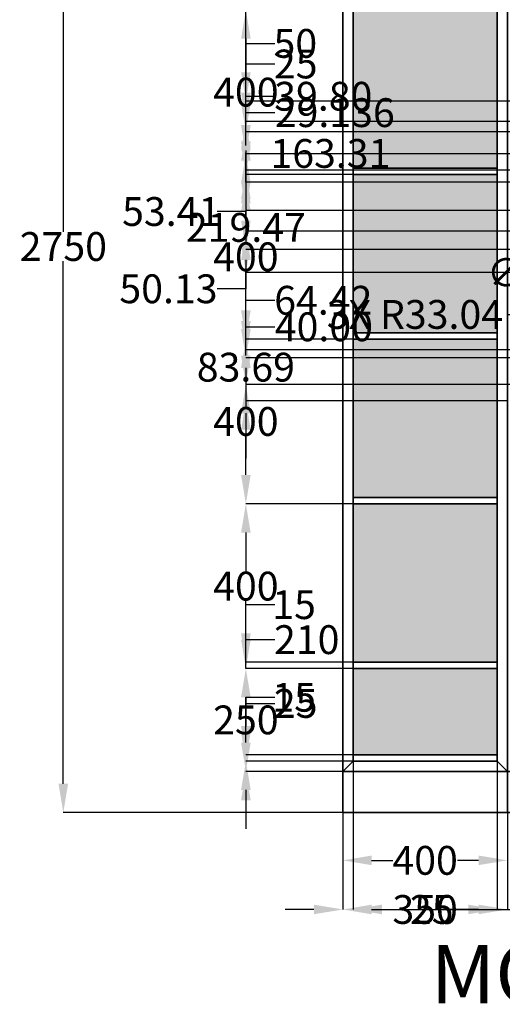
# Model space of a CAD drawing. Units: inches. Extents: x 600 to 5582, y -464 to 3142.
# Tile 1 of 9: x 600 to 1772, y -464 to 1928. Entities that reach past the tile are written whole.
import ezdxf

# ---------------------------------------------------------------- set-up
doc = ezdxf.new("R2010")
doc.units = ezdxf.units.IN
doc.header["$MEASUREMENT"] = 0
for name, color, linetype, lineweight in [('A-ANNO-DIMS', 2, 'Continuous', 18), ('A-ANNO-TEXT', 7, 'Continuous', 25), ('A-ELEV', 7, 'Continuous', 35), ('A-ELEV-PATT', 252, 'Continuous', 13)]:
    doc.layers.add(name, color=color, linetype=linetype, lineweight=lineweight)
doc.styles.get("Standard").update_dxf_attribs({"font": 'arial.ttf'})
doc.dimstyles.get("Standard").update_dxf_attribs({"dimtxt": 70, "dimasz": 70, "dimexe": 0.18, "dimexo": 0.0625, "dimgap": 0.09, "dimtad": 0, "dimtih": 1, "dimtoh": 1, "dimdec": 0, "dimzin": 0, "dimdsep": 46, "dimtxsty": 'Standard', "dimcen": 0.09, "dimadec": 0, "dimazin": 0, "dimtfac": 1, "dimtdec": 0, "dimtofl": 0, "dimtmove": 0, "dimatfit": 3, "dimfxl": 1, "dimtolj": 1, "dimtzin": 0, "dimarcsym": 0})

# ---------------------------------------------------------------- blocks, each defined once
blk = doc.blocks.new('*D1')
at = {"layer": 'A-ANNO-DIMS', "color": 0, "lineweight": -2, "transparency": 16777216}
for p, q in [((1384.7, 2752.4), (705.5, 2752.4)), ((705.7, 2682.4), (705.7, 1413.3)), ((705.7, 72.4), (705.7, 1341.6)), ((1384.7, 2.4), (705.5, 2.4))]:
    blk.add_line(p, q, dxfattribs=at)
at = {"layer": 'A-ANNO-DIMS', "color": 0, "transparency": 16777216}
for points in [[(694, 2682.4), (717.3, 2682.4), (705.7, 2752.4)], [(694, 72.4), (717.3, 72.4), (705.7, 2.4)]]:
    blk.add_solid(points, dxfattribs=at)
at = {"layer": 'Defpoints', "color": 0, "transparency": 16777216}
for p in [(1384.7, 2752.4), (705.7, 2.4), (1384.7, 2.4)]:
    blk.add_point(p, dxfattribs=at)
at = {"layer": 'A-ANNO-DIMS', "color": 0, "transparency": 16777216, "insert": (705.7, 1377.4), "char_height": 70, "attachment_point": 5}
blk.add_mtext('\\A1;2750', dxfattribs=at)
blk = doc.blocks.new('*D10')
at = {"layer": 'A-ANNO-DIMS', "color": 0, "lineweight": -2, "transparency": 16777216}
for p, q in [((1384.7, 2.4), (1384.7, -113.9)), ((1784.7, 2.4), (1784.7, -113.9)), ((1454.7, -113.8), (1506, -113.8)), ((1714.7, -113.8), (1663.5, -113.8))]:
    blk.add_line(p, q, dxfattribs=at)
at = {"layer": 'A-ANNO-DIMS', "color": 0, "transparency": 16777216}
for points in [[(1454.7, -102.1), (1454.7, -125.4), (1384.7, -113.8)], [(1714.7, -102.1), (1714.7, -125.4), (1784.7, -113.8)]]:
    blk.add_solid(points, dxfattribs=at)
at = {"layer": 'Defpoints', "color": 0, "transparency": 16777216}
for p in [(1384.7, 2.4), (1784.7, 2.4), (1784.7, -113.8)]:
    blk.add_point(p, dxfattribs=at)
at = {"layer": 'A-ANNO-DIMS', "color": 0, "transparency": 16777216, "insert": (1584.7, -113.8), "char_height": 70, "attachment_point": 5}
blk.add_mtext('\\A1;400', dxfattribs=at)
blk = doc.blocks.new('*D21')
at = {"layer": 'A-ANNO-DIMS', "color": 0, "lineweight": -2, "transparency": 16777216}
for p, q in [((1384.7, 2.4), (1384.7, -233.3)), ((4984.7, 2.4), (4984.7, -233.3)), ((1454.7, -233.1), (3080.3, -233.1)), ((4914.7, -233.1), (3289.2, -233.1))]:
    blk.add_line(p, q, dxfattribs=at)
at = {"layer": 'A-ANNO-DIMS', "color": 0, "transparency": 16777216}
for points in [[(1454.7, -221.4), (1454.7, -244.7), (1384.7, -233.1)], [(4914.7, -221.4), (4914.7, -244.7), (4984.7, -233.1)]]:
    blk.add_solid(points, dxfattribs=at)
at = {"layer": 'Defpoints', "color": 0, "transparency": 16777216}
for p in [(1384.7, 2.4), (4984.7, 2.4), (4984.7, -233.1)]:
    blk.add_point(p, dxfattribs=at)
at = {"layer": 'A-ANNO-DIMS', "color": 0, "transparency": 16777216, "insert": (3184.7, -233.1), "char_height": 70, "attachment_point": 5}
blk.add_mtext('\\A1;3600', dxfattribs=at)
blk = doc.blocks.new('*D22')
at = {"layer": 'A-ANNO-DIMS', "color": 0, "lineweight": -2, "transparency": 16777216}
for p, q in [((1149.2, 1725.8), (1149.2, 1795.8)), ((2615, 1655.8), (1149.1, 1655.8)), ((2584.7, 1602.4), (1149.1, 1602.4)), ((1149.2, 1532.4), (1149.2, 1462.4)), ((1149.2, 1462.4), (1079.2, 1462.4))]:
    blk.add_line(p, q, dxfattribs=at)
at = {"layer": 'A-ANNO-DIMS', "color": 0, "transparency": 16777216}
for points in [[(1137.6, 1725.8), (1160.9, 1725.8), (1149.2, 1655.8)], [(1137.6, 1532.4), (1160.9, 1532.4), (1149.2, 1602.4)]]:
    blk.add_solid(points, dxfattribs=at)
at = {"layer": 'Defpoints', "color": 0, "transparency": 16777216}
for p in [(2615, 1655.8), (1149.2, 1602.4), (2584.7, 1602.4)]:
    blk.add_point(p, dxfattribs=at)
at = {"layer": 'A-ANNO-DIMS', "color": 0, "transparency": 16777216, "insert": (967.8, 1462.4), "char_height": 70, "attachment_point": 5}
blk.add_mtext('\\A1;53.41', dxfattribs=at)
blk = doc.blocks.new('*D23')
at = {"layer": 'A-ANNO-DIMS', "color": 0, "lineweight": -2, "transparency": 16777216}
for p, q in [((1149.2, 1750.8), (1149.2, 1820.8)), ((1149.2, 1820.8), (1219.2, 1820.8)), ((2584.7, 1680.8), (1149.1, 1680.8)), ((2615, 1655.8), (1149.1, 1655.8)), ((1149.2, 1585.8), (1149.2, 1515.8))]:
    blk.add_line(p, q, dxfattribs=at)
at = {"layer": 'A-ANNO-DIMS', "color": 0, "transparency": 16777216}
for points in [[(1137.6, 1750.8), (1160.9, 1750.8), (1149.2, 1680.8)], [(1137.6, 1585.8), (1160.9, 1585.8), (1149.2, 1655.8)]]:
    blk.add_solid(points, dxfattribs=at)
at = {"layer": 'Defpoints', "color": 0, "transparency": 16777216}
for p in [(1149.2, 1680.8), (2584.7, 1680.8), (2615, 1655.8)]:
    blk.add_point(p, dxfattribs=at)
at = {"layer": 'A-ANNO-DIMS', "color": 0, "transparency": 16777216, "insert": (1270.3, 1820.8), "char_height": 70, "attachment_point": 5}
blk.add_mtext('\\A1;25', dxfattribs=at)
blk = doc.blocks.new('*D24')
at = {"layer": 'A-ANNO-DIMS', "color": 0, "lineweight": -2, "transparency": 16777216}
for p, q in [((1149.2, 1800.8), (1149.2, 1870.8)), ((1149.2, 1870.8), (1219.2, 1870.8)), ((2584.7, 1730.8), (1149.1, 1730.8)), ((2584.7, 1680.8), (1149.1, 1680.8)), ((1149.2, 1610.8), (1149.2, 1540.8))]:
    blk.add_line(p, q, dxfattribs=at)
at = {"layer": 'A-ANNO-DIMS', "color": 0, "transparency": 16777216}
for points in [[(1137.6, 1800.8), (1160.9, 1800.8), (1149.2, 1730.8)], [(1137.6, 1610.8), (1160.9, 1610.8), (1149.2, 1680.8)]]:
    blk.add_solid(points, dxfattribs=at)
at = {"layer": 'Defpoints', "color": 0, "transparency": 16777216}
for p in [(1149.2, 1730.8), (2584.7, 1730.8), (2584.7, 1680.8)]:
    blk.add_point(p, dxfattribs=at)
at = {"layer": 'A-ANNO-DIMS', "color": 0, "transparency": 16777216, "insert": (1269.4, 1870.8), "char_height": 70, "attachment_point": 5}
blk.add_mtext('\\A1;50', dxfattribs=at)
blk = doc.blocks.new('*D40')
at = {"layer": 'A-ANNO-DIMS', "color": 0, "lineweight": -2, "transparency": 16777216}
for p, q in [((1409.7, 352.4), (1149.1, 352.4)), ((1149.2, 282.4), (1149.2, 263.3)), ((1149.2, 172.4), (1149.2, 191.6)), ((1384.7, 102.4), (1149.1, 102.4))]:
    blk.add_line(p, q, dxfattribs=at)
at = {"layer": 'A-ANNO-DIMS', "color": 0, "transparency": 16777216}
for points in [[(1137.6, 282.4), (1160.9, 282.4), (1149.2, 352.4)], [(1137.6, 172.4), (1160.9, 172.4), (1149.2, 102.4)]]:
    blk.add_solid(points, dxfattribs=at)
at = {"layer": 'Defpoints', "color": 0, "transparency": 16777216}
for p in [(1149.2, 352.4), (1409.7, 352.4), (1384.7, 102.4)]:
    blk.add_point(p, dxfattribs=at)
at = {"layer": 'A-ANNO-DIMS', "color": 0, "transparency": 16777216, "insert": (1149.2, 227.4), "char_height": 70, "attachment_point": 5}
blk.add_mtext('\\A1;250', dxfattribs=at)
blk = doc.blocks.new('*D41')
at = {"layer": 'A-ANNO-DIMS', "color": 0, "lineweight": -2, "transparency": 16777216}
for p, q in [((1409.7, 752.4), (1149.1, 752.4)), ((1149.2, 682.4), (1149.2, 588.3)), ((1149.2, 422.4), (1149.2, 516.6)), ((1409.7, 352.4), (1149.1, 352.4))]:
    blk.add_line(p, q, dxfattribs=at)
at = {"layer": 'A-ANNO-DIMS', "color": 0, "transparency": 16777216}
for points in [[(1137.6, 682.4), (1160.9, 682.4), (1149.2, 752.4)], [(1137.6, 422.4), (1160.9, 422.4), (1149.2, 352.4)]]:
    blk.add_solid(points, dxfattribs=at)
at = {"layer": 'Defpoints', "color": 0, "transparency": 16777216}
for p in [(1149.2, 752.4), (1409.7, 752.4), (1409.7, 352.4)]:
    blk.add_point(p, dxfattribs=at)
at = {"layer": 'A-ANNO-DIMS', "color": 0, "transparency": 16777216, "insert": (1149.2, 552.4), "char_height": 70, "attachment_point": 5}
blk.add_mtext('\\A1;400', dxfattribs=at)
blk = doc.blocks.new('*D42')
at = {"layer": 'A-ANNO-DIMS', "color": 0, "lineweight": -2, "transparency": 16777216}
for p, q in [((1409.7, 1152.4), (1149.1, 1152.4)), ((1149.2, 1082.4), (1149.2, 988.3)), ((1149.2, 822.4), (1149.2, 916.6)), ((1409.7, 752.4), (1149.1, 752.4))]:
    blk.add_line(p, q, dxfattribs=at)
at = {"layer": 'A-ANNO-DIMS', "color": 0, "transparency": 16777216}
for points in [[(1137.6, 1082.4), (1160.9, 1082.4), (1149.2, 1152.4)], [(1137.6, 822.4), (1160.9, 822.4), (1149.2, 752.4)]]:
    blk.add_solid(points, dxfattribs=at)
at = {"layer": 'Defpoints', "color": 0, "transparency": 16777216}
for p in [(1149.2, 1152.4), (1409.7, 1152.4), (1409.7, 752.4)]:
    blk.add_point(p, dxfattribs=at)
at = {"layer": 'A-ANNO-DIMS', "color": 0, "transparency": 16777216, "insert": (1149.2, 952.4), "char_height": 70, "attachment_point": 5}
blk.add_mtext('\\A1;400', dxfattribs=at)
blk = doc.blocks.new('*D43')
at = {"layer": 'A-ANNO-DIMS', "color": 0, "lineweight": -2, "transparency": 16777216}
for p, q in [((1409.7, 1552.4), (1149.1, 1552.4)), ((1149.2, 1482.4), (1149.2, 1388.3)), ((1149.2, 1222.4), (1149.2, 1316.6)), ((1409.7, 1152.4), (1149.1, 1152.4))]:
    blk.add_line(p, q, dxfattribs=at)
at = {"layer": 'A-ANNO-DIMS', "color": 0, "transparency": 16777216}
for points in [[(1137.6, 1482.4), (1160.9, 1482.4), (1149.2, 1552.4)], [(1137.6, 1222.4), (1160.9, 1222.4), (1149.2, 1152.4)]]:
    blk.add_solid(points, dxfattribs=at)
at = {"layer": 'Defpoints', "color": 0, "transparency": 16777216}
for p in [(1149.2, 1552.4), (1409.7, 1552.4), (1409.7, 1152.4)]:
    blk.add_point(p, dxfattribs=at)
at = {"layer": 'A-ANNO-DIMS', "color": 0, "transparency": 16777216, "insert": (1149.2, 1352.4), "char_height": 70, "attachment_point": 5}
blk.add_mtext('\\A1;400', dxfattribs=at)
blk = doc.blocks.new('*D44')
at = {"layer": 'A-ANNO-DIMS', "color": 0, "lineweight": -2, "transparency": 16777216}
for p, q in [((1409.7, 1952.4), (1149.1, 1952.4)), ((1149.2, 1882.4), (1149.2, 1788.3)), ((1149.2, 1622.4), (1149.2, 1716.6)), ((1409.7, 1552.4), (1149.1, 1552.4))]:
    blk.add_line(p, q, dxfattribs=at)
at = {"layer": 'A-ANNO-DIMS', "color": 0, "transparency": 16777216}
for points in [[(1137.6, 1882.4), (1160.9, 1882.4), (1149.2, 1952.4)], [(1137.6, 1622.4), (1160.9, 1622.4), (1149.2, 1552.4)]]:
    blk.add_solid(points, dxfattribs=at)
at = {"layer": 'Defpoints', "color": 0, "transparency": 16777216}
for p in [(1149.2, 1952.4), (1409.7, 1952.4), (1409.7, 1552.4)]:
    blk.add_point(p, dxfattribs=at)
at = {"layer": 'A-ANNO-DIMS', "color": 0, "transparency": 16777216, "insert": (1149.2, 1752.4), "char_height": 70, "attachment_point": 5}
blk.add_mtext('\\A1;400', dxfattribs=at)
blk = doc.blocks.new('*D48')
at = {"layer": 'A-ANNO-DIMS', "color": 0, "lineweight": -2, "transparency": 16777216}
for p, q in [((1149.2, 197.4), (1149.2, 267.4)), ((1149.2, 267.4), (1219.2, 267.4)), ((1409.7, 127.4), (1149.1, 127.4)), ((1384.7, 102.4), (1149.1, 102.4)), ((1149.2, 32.4), (1149.2, -37.6))]:
    blk.add_line(p, q, dxfattribs=at)
at = {"layer": 'A-ANNO-DIMS', "color": 0, "transparency": 16777216}
for points in [[(1137.6, 197.4), (1160.9, 197.4), (1149.2, 127.4)], [(1137.6, 32.4), (1160.9, 32.4), (1149.2, 102.4)]]:
    blk.add_solid(points, dxfattribs=at)
at = {"layer": 'Defpoints', "color": 0, "transparency": 16777216}
for p in [(1149.2, 127.4), (1409.7, 127.4), (1384.7, 102.4)]:
    blk.add_point(p, dxfattribs=at)
at = {"layer": 'A-ANNO-DIMS', "color": 0, "transparency": 16777216, "insert": (1270.3, 267.4), "char_height": 70, "attachment_point": 5}
blk.add_mtext('\\A1;25', dxfattribs=at)
blk = doc.blocks.new('*D49')
at = {"layer": 'A-ANNO-DIMS', "color": 0, "lineweight": -2, "transparency": 16777216}
for p, q in [((1149.2, 212.4), (1149.2, 282.4)), ((1149.2, 282.4), (1219.2, 282.4)), ((1409.7, 142.4), (1149.1, 142.4)), ((1409.7, 127.4), (1149.1, 127.4)), ((1149.2, 57.4), (1149.2, -12.6))]:
    blk.add_line(p, q, dxfattribs=at)
at = {"layer": 'A-ANNO-DIMS', "color": 0, "transparency": 16777216}
for points in [[(1137.6, 212.4), (1160.9, 212.4), (1149.2, 142.4)], [(1137.6, 57.4), (1160.9, 57.4), (1149.2, 127.4)]]:
    blk.add_solid(points, dxfattribs=at)
at = {"layer": 'Defpoints', "color": 0, "transparency": 16777216}
for p in [(1149.2, 142.4), (1409.7, 142.4), (1409.7, 127.4)]:
    blk.add_point(p, dxfattribs=at)
at = {"layer": 'A-ANNO-DIMS', "color": 0, "transparency": 16777216, "insert": (1266.4, 282.4), "char_height": 70, "attachment_point": 5}
blk.add_mtext('\\A1;15', dxfattribs=at)
blk = doc.blocks.new('*D50')
at = {"layer": 'A-ANNO-DIMS', "color": 0, "lineweight": -2, "transparency": 16777216}
for p, q in [((1149.2, 352.4), (1149.2, 422.4)), ((1149.2, 422.4), (1219.2, 422.4)), ((1409.7, 352.4), (1149.1, 352.4)), ((1149.2, 212.4), (1149.2, 282.4)), ((1409.7, 142.4), (1149.1, 142.4))]:
    blk.add_line(p, q, dxfattribs=at)
at = {"layer": 'A-ANNO-DIMS', "color": 0, "transparency": 16777216}
for points in [[(1137.6, 282.4), (1160.9, 282.4), (1149.2, 352.4)], [(1137.6, 212.4), (1160.9, 212.4), (1149.2, 142.4)]]:
    blk.add_solid(points, dxfattribs=at)
at = {"layer": 'Defpoints', "color": 0, "transparency": 16777216}
for p in [(1149.2, 352.4), (1409.7, 352.4), (1409.7, 142.4)]:
    blk.add_point(p, dxfattribs=at)
at = {"layer": 'A-ANNO-DIMS', "color": 0, "transparency": 16777216, "insert": (1297.1, 422.4), "char_height": 70, "attachment_point": 5}
blk.add_mtext('\\A1;210', dxfattribs=at)
blk = doc.blocks.new('*D51')
at = {"layer": 'A-ANNO-DIMS', "color": 0, "lineweight": -2, "transparency": 16777216}
for p, q in [((1149.2, 437.4), (1149.2, 507.4)), ((1149.2, 507.4), (1219.2, 507.4)), ((1409.7, 367.4), (1149.1, 367.4)), ((1409.7, 352.4), (1149.1, 352.4)), ((1149.2, 282.4), (1149.2, 212.4))]:
    blk.add_line(p, q, dxfattribs=at)
at = {"layer": 'A-ANNO-DIMS', "color": 0, "transparency": 16777216}
for points in [[(1137.6, 437.4), (1160.9, 437.4), (1149.2, 367.4)], [(1137.6, 282.4), (1160.9, 282.4), (1149.2, 352.4)]]:
    blk.add_solid(points, dxfattribs=at)
at = {"layer": 'Defpoints', "color": 0, "transparency": 16777216}
for p in [(1149.2, 367.4), (1409.7, 367.4), (1409.7, 352.4)]:
    blk.add_point(p, dxfattribs=at)
at = {"layer": 'A-ANNO-DIMS', "color": 0, "transparency": 16777216, "insert": (1266.4, 507.4), "char_height": 70, "attachment_point": 5}
blk.add_mtext('\\A1;15', dxfattribs=at)
blk = doc.blocks.new('*D52')
at = {"layer": 'A-ANNO-DIMS', "color": 0, "lineweight": -2, "transparency": 16777216}
for p, q in [((1409.7, 127.4), (1409.7, -233.3)), ((1384.7, 102.4), (1384.7, -233.3)), ((1314.7, -233.1), (1244.7, -233.1)), ((1479.7, -233.1), (1549.7, -233.1))]:
    blk.add_line(p, q, dxfattribs=at)
at = {"layer": 'A-ANNO-DIMS', "color": 0, "transparency": 16777216}
for points in [[(1314.7, -221.4), (1314.7, -244.7), (1384.7, -233.1)], [(1479.7, -221.4), (1479.7, -244.7), (1409.7, -233.1)]]:
    blk.add_solid(points, dxfattribs=at)
at = {"layer": 'Defpoints', "color": 0, "transparency": 16777216}
for p in [(1409.7, 127.4), (1384.7, 102.4), (1409.7, -233.1)]:
    blk.add_point(p, dxfattribs=at)
at = {"layer": 'A-ANNO-DIMS', "color": 0, "transparency": 16777216, "insert": (1600.8, -233.1), "char_height": 70, "attachment_point": 5}
blk.add_mtext('\\A1;25', dxfattribs=at)
blk = doc.blocks.new('*D53')
at = {"layer": 'A-ANNO-DIMS', "color": 0, "lineweight": -2, "transparency": 16777216}
for p, q in [((1409.7, 127.4), (1409.7, -233.3)), ((1759.7, 127.4), (1759.7, -233.3)), ((1479.7, -233.1), (1507.5, -233.1)), ((1689.7, -233.1), (1662, -233.1))]:
    blk.add_line(p, q, dxfattribs=at)
at = {"layer": 'A-ANNO-DIMS', "color": 0, "transparency": 16777216}
for points in [[(1479.7, -221.4), (1479.7, -244.7), (1409.7, -233.1)], [(1689.7, -221.4), (1689.7, -244.7), (1759.7, -233.1)]]:
    blk.add_solid(points, dxfattribs=at)
at = {"layer": 'Defpoints', "color": 0, "transparency": 16777216}
for p in [(1409.7, 127.4), (1759.7, 127.4), (1759.7, -233.1)]:
    blk.add_point(p, dxfattribs=at)
at = {"layer": 'A-ANNO-DIMS', "color": 0, "transparency": 16777216, "insert": (1584.7, -233.1), "char_height": 70, "attachment_point": 5}
blk.add_mtext('\\A1;350', dxfattribs=at)
blk = doc.blocks.new('*D54')
at = {"layer": 'A-ANNO-DIMS', "color": 0, "lineweight": -2, "transparency": 16777216}
for p, q in [((1759.7, 127.4), (1759.7, -233.3)), ((1784.7, 102.4), (1784.7, -233.3)), ((1689.7, -233.1), (1619.7, -233.1)), ((1854.7, -233.1), (1924.7, -233.1))]:
    blk.add_line(p, q, dxfattribs=at)
at = {"layer": 'A-ANNO-DIMS', "color": 0, "transparency": 16777216}
for points in [[(1689.7, -221.4), (1689.7, -244.7), (1759.7, -233.1)], [(1854.7, -221.4), (1854.7, -244.7), (1784.7, -233.1)]]:
    blk.add_solid(points, dxfattribs=at)
at = {"layer": 'Defpoints', "color": 0, "transparency": 16777216}
for p in [(1759.7, 127.4), (1784.7, 102.4), (1784.7, -233.1)]:
    blk.add_point(p, dxfattribs=at)
at = {"layer": 'A-ANNO-DIMS', "color": 0, "transparency": 16777216, "insert": (1975.8, -233.1), "char_height": 70, "attachment_point": 5}
blk.add_mtext('\\A1;25', dxfattribs=at)
blk = doc.blocks.new('*D55')
at = {"layer": 'A-ANNO-DIMS', "color": 0, "lineweight": -2, "transparency": 16777216}
for p, q in [((1784.7, 102.4), (1784.7, -233.3)), ((1884.7, 102.4), (1884.7, -233.3)), ((1714.7, -233.1), (1644.7, -233.1)), ((1954.7, -233.1), (2024.7, -233.1))]:
    blk.add_line(p, q, dxfattribs=at)
at = {"layer": 'A-ANNO-DIMS', "color": 0, "transparency": 16777216}
for points in [[(1714.7, -221.4), (1714.7, -244.7), (1784.7, -233.1)], [(1954.7, -221.4), (1954.7, -244.7), (1884.7, -233.1)]]:
    blk.add_solid(points, dxfattribs=at)
at = {"layer": 'Defpoints', "color": 0, "transparency": 16777216}
for p in [(1784.7, 102.4), (1884.7, 102.4), (1884.7, -233.1)]:
    blk.add_point(p, dxfattribs=at)
at = {"layer": 'A-ANNO-DIMS', "color": 0, "transparency": 16777216, "insert": (2098.8, -233.1), "char_height": 70, "attachment_point": 5}
blk.add_mtext('\\A1;100', dxfattribs=at)
blk = doc.blocks.new('*D63')
at = {"layer": 'A-ANNO-DIMS', "color": 0, "lineweight": -2, "transparency": 16777216}
for p, q in [((2584.7, 2352.4), (1149.1, 2352.4)), ((1149.2, 2282.4), (1149.2, 2077.5)), ((1149.2, 1800.8), (1149.2, 2005.8)), ((2584.7, 1730.8), (1149.1, 1730.8))]:
    blk.add_line(p, q, dxfattribs=at)
at = {"layer": 'A-ANNO-DIMS', "color": 0, "transparency": 16777216}
for points in [[(1137.6, 2282.4), (1160.9, 2282.4), (1149.2, 2352.4)], [(1137.6, 1800.8), (1160.9, 1800.8), (1149.2, 1730.8)]]:
    blk.add_solid(points, dxfattribs=at)
at = {"layer": 'Defpoints', "color": 0, "transparency": 16777216}
for p in [(1149.2, 2352.4), (2584.7, 2352.4), (2584.7, 1730.8)]:
    blk.add_point(p, dxfattribs=at)
at = {"layer": 'A-ANNO-DIMS', "color": 0, "transparency": 16777216, "insert": (1149.2, 2041.6), "char_height": 70, "attachment_point": 5}
blk.add_mtext('\\A1;621.59', dxfattribs=at)
blk = doc.blocks.new('*D65')
at = {"layer": 'A-ANNO-DIMS', "color": 0, "lineweight": -2, "transparency": 16777216}
for p, q in [((1784.7, 2352.4), (1784.7, -233.3)), ((2184.7, 2352.4), (2184.7, -233.3)), ((1714.7, -233.1), (1644.7, -233.1)), ((2254.7, -233.1), (2324.7, -233.1))]:
    blk.add_line(p, q, dxfattribs=at)
at = {"layer": 'A-ANNO-DIMS', "color": 0, "transparency": 16777216}
for points in [[(1714.7, -221.4), (1714.7, -244.7), (1784.7, -233.1)], [(2254.7, -221.4), (2254.7, -244.7), (2184.7, -233.1)]]:
    blk.add_solid(points, dxfattribs=at)
at = {"layer": 'Defpoints', "color": 0, "transparency": 16777216}
for p in [(1784.7, 2352.4), (2184.7, 2352.4), (2184.7, -233.1)]:
    blk.add_point(p, dxfattribs=at)
at = {"layer": 'A-ANNO-DIMS', "color": 0, "transparency": 16777216, "insert": (1984.7, -233.1), "char_height": 70, "attachment_point": 5}
blk.add_mtext('\\A1;400.00', dxfattribs=at)
blk = doc.blocks.new('*D70')
at = {"layer": 'A-ANNO-DIMS', "color": 0, "lineweight": -2, "transparency": 16777216}
for p, q in [((1149.2, 1176.8), (1149.2, 1246.8)), ((1149.2, 1246.8), (1219.2, 1246.8)), ((2586.9, 1106.8), (1149.1, 1106.8)), ((2599.2, 1042.4), (1149.1, 1042.4)), ((1149.2, 972.4), (1149.2, 902.4))]:
    blk.add_line(p, q, dxfattribs=at)
at = {"layer": 'A-ANNO-DIMS', "color": 0, "transparency": 16777216}
for points in [[(1137.6, 1176.8), (1160.9, 1176.8), (1149.2, 1106.8)], [(1137.6, 972.4), (1160.9, 972.4), (1149.2, 1042.4)]]:
    blk.add_solid(points, dxfattribs=at)
at = {"layer": 'Defpoints', "color": 0, "transparency": 16777216}
for p in [(1149.2, 1106.8), (2586.9, 1106.8), (2599.2, 1042.4)]:
    blk.add_point(p, dxfattribs=at)
at = {"layer": 'A-ANNO-DIMS', "color": 0, "transparency": 16777216, "insert": (1337.3, 1246.8), "char_height": 70, "attachment_point": 5}
blk.add_mtext('\\A1;64.42', dxfattribs=at)
blk = doc.blocks.new('*D76')
at = {"layer": 'A-ANNO-DIMS', "color": 0, "lineweight": -2, "transparency": 16777216}
for p, q in [((1149.2, 1112.4), (1149.2, 1182.4)), ((1149.2, 1182.4), (1219.2, 1182.4)), ((1784.7, 1042.4), (1149.1, 1042.4)), ((1784.7, 1002.4), (1149.1, 1002.4)), ((1149.2, 932.4), (1149.2, 862.4))]:
    blk.add_line(p, q, dxfattribs=at)
at = {"layer": 'A-ANNO-DIMS', "color": 0, "transparency": 16777216}
for points in [[(1137.6, 1112.4), (1160.9, 1112.4), (1149.2, 1042.4)], [(1137.6, 932.4), (1160.9, 932.4), (1149.2, 1002.4)]]:
    blk.add_solid(points, dxfattribs=at)
at = {"layer": 'Defpoints', "color": 0, "transparency": 16777216}
for p in [(1149.2, 1042.4), (1784.7, 1042.4), (1784.7, 1002.4)]:
    blk.add_point(p, dxfattribs=at)
at = {"layer": 'A-ANNO-DIMS', "color": 0, "transparency": 16777216, "insert": (1338.7, 1182.4), "char_height": 70, "attachment_point": 5}
blk.add_mtext('\\A1;40.00', dxfattribs=at)
blk = doc.blocks.new('*D80')
at = {"layer": 'A-ANNO-DIMS', "color": 0, "lineweight": -2, "transparency": 16777216}
for p, q in [((1149.2, 1196.1), (1149.2, 1266.1)), ((1925.6, 1126.1), (1149.1, 1126.1)), ((1925.6, 1042.4), (1149.1, 1042.4)), ((1149.2, 972.4), (1149.2, 902.4))]:
    blk.add_line(p, q, dxfattribs=at)
at = {"layer": 'A-ANNO-DIMS', "color": 0, "transparency": 16777216}
for points in [[(1137.6, 1196.1), (1160.9, 1196.1), (1149.2, 1126.1)], [(1137.6, 972.4), (1160.9, 972.4), (1149.2, 1042.4)]]:
    blk.add_solid(points, dxfattribs=at)
at = {"layer": 'Defpoints', "color": 0, "transparency": 16777216}
for p in [(1149.2, 1126.1), (1925.7, 1126.1), (1925.7, 1042.4)]:
    blk.add_point(p, dxfattribs=at)
at = {"layer": 'A-ANNO-DIMS', "color": 0, "transparency": 16777216, "insert": (1149.2, 1084.3), "char_height": 70, "attachment_point": 5}
blk.add_mtext('\\A1;83.69', dxfattribs=at)
blk = doc.blocks.new('*D86')
at = {"layer": 'A-ANNO-DIMS', "color": 0, "lineweight": -2, "transparency": 16777216}
for p, q in [((1714.7, 2987.9), (1644.7, 2987.9)), ((1784.7, 1602.5), (1784.7, 2988.1)), ((1877.2, 1562.7), (1877.2, 2988.1)), ((1947.2, 2987.9), (2017.2, 2987.9))]:
    blk.add_line(p, q, dxfattribs=at)
at = {"layer": 'A-ANNO-DIMS', "color": 0, "transparency": 16777216}
for points in [[(1714.7, 2999.6), (1714.7, 2976.3), (1784.7, 2987.9)], [(1947.2, 2999.6), (1947.2, 2976.3), (1877.2, 2987.9)]]:
    blk.add_solid(points, dxfattribs=at)
at = {"layer": 'Defpoints', "color": 0, "transparency": 16777216}
for p in [(1877.2, 2987.9), (1784.7, 1602.4), (1877.2, 1562.6)]:
    blk.add_point(p, dxfattribs=at)
at = {"layer": 'A-ANNO-DIMS', "color": 0, "transparency": 16777216, "insert": (2135.4, 2987.9), "char_height": 70, "attachment_point": 5}
blk.add_mtext('\\A1;92.46', dxfattribs=at)
blk = doc.blocks.new('*D87')
at = {"layer": 'A-ANNO-DIMS', "color": 0, "lineweight": -2, "transparency": 16777216}
for p, q in [((1149.2, 1672.4), (1149.2, 1742.4)), ((1149.2, 1742.4), (1219.2, 1742.4)), ((1784.7, 1602.4), (1149.1, 1602.4)), ((1877.1, 1562.6), (1149.1, 1562.6)), ((1149.2, 1492.6), (1149.2, 1422.6))]:
    blk.add_line(p, q, dxfattribs=at)
at = {"layer": 'A-ANNO-DIMS', "color": 0, "transparency": 16777216}
for points in [[(1137.6, 1672.4), (1160.9, 1672.4), (1149.2, 1602.4)], [(1137.6, 1492.6), (1160.9, 1492.6), (1149.2, 1562.6)]]:
    blk.add_solid(points, dxfattribs=at)
at = {"layer": 'Defpoints', "color": 0, "transparency": 16777216}
for p in [(1149.2, 1602.4), (1784.7, 1602.4), (1877.2, 1562.6)]:
    blk.add_point(p, dxfattribs=at)
at = {"layer": 'A-ANNO-DIMS', "color": 0, "transparency": 16777216, "insert": (1337.3, 1742.4), "char_height": 70, "attachment_point": 5}
blk.add_mtext('\\A1;39.80', dxfattribs=at)
blk = doc.blocks.new('*D88')
at = {"layer": 'A-ANNO-DIMS', "color": 0, "lineweight": -2, "transparency": 16777216}
for p, q in [((1149.2, 1632.6), (1149.2, 1702.6)), ((1149.2, 1702.6), (1219.2, 1702.6)), ((1877.1, 1562.6), (1149.1, 1562.6)), ((1877.1, 1533.5), (1149.1, 1533.5)), ((1149.2, 1463.5), (1149.2, 1393.5))]:
    blk.add_line(p, q, dxfattribs=at)
at = {"layer": 'A-ANNO-DIMS', "color": 0, "transparency": 16777216}
for points in [[(1137.6, 1632.6), (1160.9, 1632.6), (1149.2, 1562.6)], [(1137.6, 1463.5), (1160.9, 1463.5), (1149.2, 1533.5)]]:
    blk.add_solid(points, dxfattribs=at)
at = {"layer": 'Defpoints', "color": 0, "transparency": 16777216}
for p in [(1149.2, 1562.6), (1877.2, 1562.6), (1877.2, 1533.5)]:
    blk.add_point(p, dxfattribs=at)
at = {"layer": 'A-ANNO-DIMS', "color": 0, "transparency": 16777216, "insert": (1365.2, 1702.6), "char_height": 70, "attachment_point": 5}
blk.add_mtext('\\A1;29.136', dxfattribs=at)
blk = doc.blocks.new('*D89')
at = {"layer": 'A-ANNO-DIMS', "color": 0, "lineweight": -2, "transparency": 16777216}
for p, q in [((1807.2, 2987.9), (1737.2, 2987.9)), ((1877.2, 1533.5), (1877.2, 2988.1)), ((1925.6, 1533.5), (1925.6, 2988.1)), ((1995.6, 2987.9), (2065.6, 2987.9))]:
    blk.add_line(p, q, dxfattribs=at)
at = {"layer": 'A-ANNO-DIMS', "color": 0, "transparency": 16777216}
for points in [[(1807.2, 2999.6), (1807.2, 2976.3), (1877.2, 2987.9)], [(1995.6, 2999.6), (1995.6, 2976.3), (1925.6, 2987.9)]]:
    blk.add_solid(points, dxfattribs=at)
at = {"layer": 'Defpoints', "color": 0, "transparency": 16777216}
for p in [(1925.6, 2987.9), (1877.2, 1533.5), (1925.6, 1533.5)]:
    blk.add_point(p, dxfattribs=at)
at = {"layer": 'A-ANNO-DIMS', "color": 0, "transparency": 16777216, "insert": (2185.1, 2987.9), "char_height": 70, "attachment_point": 5}
blk.add_mtext('\\A1;48.40', dxfattribs=at)
blk = doc.blocks.new('*D97')
at = {"layer": 'A-ANNO-DIMS', "color": 0, "lineweight": -2, "transparency": 16777216}
for p, q in [((1149.2, 1533.5), (1149.2, 1603.5)), ((1149.2, 1603.5), (1219.2, 1603.5)), ((1925.5, 1533.5), (1149.1, 1533.5)), ((1149.2, 1440.2), (1149.2, 1463.5)), ((1925.5, 1370.2), (1149.1, 1370.2))]:
    blk.add_line(p, q, dxfattribs=at)
at = {"layer": 'A-ANNO-DIMS', "color": 0, "transparency": 16777216}
for points in [[(1137.6, 1463.5), (1160.9, 1463.5), (1149.2, 1533.5)], [(1137.6, 1440.2), (1160.9, 1440.2), (1149.2, 1370.2)]]:
    blk.add_solid(points, dxfattribs=at)
at = {"layer": 'Defpoints', "color": 0, "transparency": 16777216}
for p in [(1149.2, 1533.5), (1925.6, 1533.5), (1925.6, 1370.2)]:
    blk.add_point(p, dxfattribs=at)
at = {"layer": 'A-ANNO-DIMS', "color": 0, "transparency": 16777216, "insert": (1354.6, 1603.5), "char_height": 70, "attachment_point": 5}
blk.add_mtext('\\A1;163.31', dxfattribs=at)
blk = doc.blocks.new('*D98')
at = {"layer": 'A-ANNO-DIMS', "color": 0, "lineweight": -2, "transparency": 16777216}
for p, q in [((2213.4, 1533.5), (1149.1, 1533.5)), ((1149.2, 1463.5), (1149.2, 1459.6)), ((1149.2, 1384), (1149.2, 1387.9)), ((2210.8, 1314), (1149.1, 1314))]:
    blk.add_line(p, q, dxfattribs=at)
at = {"layer": 'A-ANNO-DIMS', "color": 0, "transparency": 16777216}
for points in [[(1137.6, 1463.5), (1160.9, 1463.5), (1149.2, 1533.5)], [(1137.6, 1384), (1160.9, 1384), (1149.2, 1314)]]:
    blk.add_solid(points, dxfattribs=at)
at = {"layer": 'Defpoints', "color": 0, "transparency": 16777216}
for p in [(2213.5, 1533.5), (1149.2, 1314), (2210.8, 1314)]:
    blk.add_point(p, dxfattribs=at)
at = {"layer": 'A-ANNO-DIMS', "color": 0, "transparency": 16777216, "insert": (1149.2, 1423.8), "char_height": 70, "attachment_point": 5}
blk.add_mtext('\\A1;219.47', dxfattribs=at)
blk = doc.blocks.new('*D101')
at = {"layer": 'A-ANNO-DIMS', "color": 0, "lineweight": -2, "transparency": 16777216}
for p, q in [((1149.2, 1534.8), (1149.2, 1604.8)), ((2272.8, 1464.8), (1149.1, 1464.8)), ((2272.8, 1414.7), (1149.1, 1414.7)), ((1149.2, 1344.7), (1149.2, 1274.7)), ((1149.2, 1274.7), (1079.2, 1274.7))]:
    blk.add_line(p, q, dxfattribs=at)
at = {"layer": 'A-ANNO-DIMS', "color": 0, "transparency": 16777216}
for points in [[(1137.6, 1534.8), (1160.9, 1534.8), (1149.2, 1464.8)], [(1137.6, 1344.7), (1160.9, 1344.7), (1149.2, 1414.7)]]:
    blk.add_solid(points, dxfattribs=at)
at = {"layer": 'Defpoints', "color": 0, "transparency": 16777216}
for p in [(2272.9, 1464.8), (1149.2, 1414.7), (2272.9, 1414.7)]:
    blk.add_point(p, dxfattribs=at)
at = {"layer": 'A-ANNO-DIMS', "color": 0, "transparency": 16777216, "insert": (961.1, 1274.7), "char_height": 70, "attachment_point": 5}
blk.add_mtext('\\A1;50.13', dxfattribs=at)
blk = doc.blocks.new('*D104')
at = {"layer": 'A-ANNO-DIMS', "color": 0, "lineweight": -2, "transparency": 16777216}
for p, q in [((1786.6, 1212.4), (1856.6, 1212.4)), ((1856.6, 1212.4), (1916.6, 1176.4)), ((2004.9, 1123.3), (2005.1, 1123.3)), ((2005, 1123.3), (2005, 1123.4))]:
    blk.add_line(p, q, dxfattribs=at)
at = {"layer": 'A-ANNO-DIMS', "color": 0, "transparency": 16777216}
blk.add_solid([(1922.6, 1186.4), (1910.6, 1166.4), (1976.6, 1140.4)], dxfattribs=at)
at = {"layer": 'Defpoints', "color": 0, "transparency": 16777216}
for p in [(1976.6, 1140.4), (2005, 1123.3)]:
    blk.add_point(p, dxfattribs=at)
at = {"layer": 'A-ANNO-DIMS', "color": 0, "transparency": 16777216, "insert": (1559.9, 1212.4), "char_height": 70, "attachment_point": 5}
blk.add_mtext('\\A1;3X R33.04', dxfattribs=at)
blk = doc.blocks.new('*D106')
at = {"layer": 'A-ANNO-DIMS', "color": 0, "lineweight": -2, "transparency": 16777216}
for p, q in [((2057.7, 1313.8), (2127.7, 1313.9)), ((2210.7, 1314), (2210.9, 1314)), ((2210.8, 1313.9), (2210.8, 1314.1))]:
    blk.add_line(p, q, dxfattribs=at)
at = {"layer": 'A-ANNO-DIMS', "color": 0, "transparency": 16777216}
blk.add_solid([(2127.7, 1325.5), (2127.7, 1302.2), (2197.7, 1314)], dxfattribs=at)
at = {"layer": 'Defpoints', "color": 0, "transparency": 16777216}
for p in [(2197.7, 1314), (2224, 1314)]:
    blk.add_point(p, dxfattribs=at)
at = {"layer": 'A-ANNO-DIMS', "color": 0, "transparency": 16777216, "insert": (1901.4, 1313.8), "char_height": 70, "attachment_point": 5}
blk.add_mtext('\\A1;∅26.33', dxfattribs=at)

msp = doc.modelspace()

# ---------------------------------------------------------------- hatches: boundary and pattern name
at = {"layer": 'A-ELEV-PATT'}
h = msp.add_hatch(dxfattribs=at)
h.set_pattern_fill('CROSS', color=256, scale=100)
h.paths.add_polyline_path([(1759.7485, 2327.4212), (1409.7485, 2327.4212), (1409.7485, 1967.4212), (1759.7485, 1967.4212)])
h.paths.add_polyline_path([(1759.7485, 1952.4212), (1409.7485, 1952.4212), (1409.7485, 1567.4212), (1759.7485, 1567.4212)])
h.paths.add_polyline_path([(1759.7485, 1552.4212), (1409.7485, 1552.4212), (1409.7485, 1167.4212), (1759.7485, 1167.4212)])
h.paths.add_polyline_path([(1759.7485, 1152.4212), (1409.7485, 1152.4212), (1409.7485, 767.4212), (1759.7485, 767.4212)])
h.paths.add_polyline_path([(1759.7485, 752.4212), (1409.7485, 752.4212), (1409.7485, 367.4212), (1759.7485, 367.4212)])
h.paths.add_polyline_path([(1759.7485, 352.4212), (1409.7485, 352.4212), (1409.7485, 142.4212), (1759.7485, 142.4212)])
h.paths.add_polyline_path([(3759.7485, 1977.4212), (3409.7485, 1977.4212), (3409.7485, 1627.4212), (3759.7485, 1627.4212)])
h.paths.add_polyline_path([(3714.7508, 1954.858, -1), (3750.8891, 1954.858, -1)], flags=16)
h.paths.add_polyline_path([(3759.7485, 2327.4212), (3409.7485, 2327.4212), (3409.7485, 2002.4212), (3759.7485, 2002.4212)])
h.paths.add_polyline_path([(4159.7485, 2327.4212), (3809.7485, 2327.4212), (3809.7485, 2002.4212), (4159.7485, 2002.4212)])
h.paths.add_polyline_path([(4159.7485, 1977.4212), (3809.7485, 1977.4212), (3813.5467, 1954.858, -1), (3849.685, 1954.858, -1), (3813.5467, 1954.858), (3809.7485, 1627.4212), (4159.7485, 1627.4212)])
h.paths.add_polyline_path([(4559.7485, 2327.4212), (4184.7485, 2327.4212), (4184.7485, 2002.4212), (4559.7485, 2002.4212)])
h.paths.add_polyline_path([(4559.7485, 1977.4212), (4184.7485, 1977.4212), (4184.7485, 1627.4212), (4559.7485, 1627.4212)])
h.paths.add_polyline_path([(4517.0704, 1954.858, -1), (4553.2087, 1954.858, -1)], flags=16)
h.paths.add_polyline_path([(4959.7485, 2327.4212), (4609.7485, 2327.4212), (4609.7485, 2002.4212), (4959.7485, 2002.4212)])
h.paths.add_polyline_path([(4959.7485, 1977.4212), (4609.7485, 1977.4212), (4609.7485, 1627.4212), (4959.7485, 1627.4212)])
h.paths.add_polyline_path([(4619.5464, 1954.858, -1), (4655.6847, 1954.858, -1)], flags=16)

# ---------------------------------------------------------------- linework, layer by layer
at = {"layer": 'A-ELEV'}
for p, q in [((1409.7485, 1567.4212), (1759.7485, 1567.4212)), ((1409.7485, 1552.4212), (1759.7485, 1552.4212)), ((1409.7485, 1167.4212), (1759.7485, 1167.4212)), ((1409.7485, 1152.4212), (1759.7485, 1152.4212)), ((1409.7485, 767.4212), (1759.7485, 767.4212)), ((1409.7485, 752.4212), (1759.7485, 752.4212)), ((1409.7485, 367.4212), (1759.7485, 367.4212)), ((1409.7485, 352.4212), (1759.7485, 352.4212)), ((1409.7485, 142.4212), (1759.7485, 142.4212)), ((4984.7485, 102.4212), (1384.7485, 102.4212))]:
    msp.add_line(p, q, dxfattribs=at)
for points in [[(4984.7485, 2.4212), (4984.7485, 2752.4212), (1384.7485, 2752.4212), (1384.7485, 2.4212)], [(1384.7485, 102.4212), (1409.7485, 127.4212), (1759.7485, 127.4212), (1784.7485, 102.4212)]]:
    msp.add_lwpolyline(points, close=True, dxfattribs=at)
for points in [[(1784.7485, 2.4212), (1784.7485, 2352.4212), (1384.7485, 2352.4212), (1409.7485, 2327.4212), (1759.7485, 2327.4212), (1409.7485, 2327.4212), (1409.7485, 127.4212)], [(1759.7485, 127.4212), (1759.7485, 2327.4212), (1784.7485, 2352.4212), (2184.7485, 2352.4212), (2184.7485, 1602.4212)]]:
    msp.add_lwpolyline(points, dxfattribs=at)

# ---------------------------------------------------------------- texts
at = {"layer": 'A-ANNO-TEXT'}
msp.add_text('MODULAR KITCHEN ELEVATION', height=141.903549, dxfattribs=at).set_placement((1598.0156, -460.987))

# ---------------------------------------------------------------- dimensions: what is measured, and where the dimension line sits
at = {"layer": 'A-ANNO-DIMS'}
for base, p1, p2, override, picture, middle in [((1877.2057, 2987.9212), (1784.7485, 1602.4212), (1877.2057, 1562.623), {"dimdec": 2, "dimlfac": 1, "dimrnd": 0, "dimzin": 0, "dimdsep": 46, "dimlunit": 2}, '*D86', (2135.3789, 2987.9212)), ((1925.6025, 2987.9212), (1877.2057, 1533.4874), (1925.6025, 1533.4874), {"dimdec": 2, "dimlfac": 1, "dimrnd": 0, "dimzin": 0, "dimdsep": 46, "dimlunit": 2}, '*D89', (2185.0889, 2987.9212)), ((2184.7485, -233.0788), (1784.7485, 2352.4212), (2184.7485, 2352.4212), {"dimdec": 2, "dimlfac": 1, "dimrnd": 0, "dimzin": 0, "dimdsep": 46, "dimlunit": 2}, '*D65', (1984.7485, -233.0788)), ((1409.7485, -233.0788), (1384.7485, 102.4212), (1409.7485, 127.4212), {"dimdec": 0, "dimlfac": 1, "dimrnd": 0, "dimzin": 0, "dimdsep": 46, "dimlunit": 2}, '*D52', (1600.8344, -233.0788)), ((1759.7485, -233.0788), (1409.7485, 127.4212), (1759.7485, 127.4212), {"dimdec": 0, "dimlfac": 1, "dimrnd": 0, "dimzin": 0, "dimdsep": 46, "dimlunit": 2}, '*D53', (1584.7485, -233.0788)), ((1784.7485, -233.0788), (1759.7485, 127.4212), (1784.7485, 102.4212), {"dimdec": 0, "dimlfac": 1, "dimrnd": 0, "dimzin": 0, "dimdsep": 46, "dimlunit": 2}, '*D54', (1975.8344, -233.0788)), ((1884.7485, -233.0788), (1784.7485, 102.4212), (1884.7485, 102.4212), {"dimdec": 0, "dimlfac": 1, "dimrnd": 0, "dimzin": 0, "dimdsep": 46, "dimlunit": 2}, '*D55', (2098.7539, -233.0788)), ((1784.7485, -113.7624), (1384.7485, 2.4212), (1784.7485, 2.4212), {"dimclrd": 0, "dimclre": 0, "dimclrt": 0}, '*D10', (1584.7485, -113.7624)), ((4984.7485, -233.0788), (1384.7485, 2.4212), (4984.7485, 2.4212), {"dimdec": 0, "dimlfac": 1, "dimrnd": 0, "dimzin": 0, "dimdsep": 46, "dimlunit": 2}, '*D21', (3184.7485, -233.0788))]:
    dim = msp.add_linear_dim(base=base, p1=p1, p2=p2, dimstyle='Standard', override=override, dxfattribs=at)
    dim.commit()
    dim.dimension.update_dxf_attribs({"geometry": picture, "text_midpoint": middle})
for base, p1, p2, override, picture, middle in [((705.6833, 2.4212), (1384.7485, 2752.4212), (1384.7485, 2.4212), {"dimclrd": 0, "dimclre": 0, "dimclrt": 0}, '*D1', (705.6833, 1377.4212)), ((1149.2485, 2352.4212), (2584.7485, 1730.8271), (2584.7485, 2352.4212), {"dimdec": 2, "dimlfac": 1, "dimrnd": 0, "dimzin": 0, "dimdsep": 46, "dimlunit": 2}, '*D63', (1149.2485, 2041.6241)), ((1149.2485, 1952.4212), (1409.7485, 1552.4212), (1409.7485, 1952.4212), {"dimdec": 0, "dimlfac": 1, "dimrnd": 0, "dimzin": 0, "dimdsep": 46, "dimlunit": 2}, '*D44', (1149.2485, 1752.4212)), ((1149.2485, 1730.8271), (2584.7485, 1680.8271), (2584.7485, 1730.8271), {"dimdec": 0, "dimlfac": 1, "dimrnd": 0, "dimzin": 0, "dimdsep": 46, "dimlunit": 2}, '*D24', (1269.3555, 1870.8271)), ((1149.2485, 1680.8271), (2615.026, 1655.8271), (2584.7485, 1680.8271), {"dimdec": 0, "dimlfac": 1, "dimrnd": 0, "dimzin": 0, "dimdsep": 46, "dimlunit": 2}, '*D23', (1270.3344, 1820.8271)), ((1149.2485, 1602.4212), (2615.026, 1655.8271), (2584.7485, 1602.4212), {"dimdec": 2, "dimlfac": 1, "dimrnd": 0, "dimzin": 0, "dimdsep": 46, "dimlunit": 2}, '*D22', (967.8079, 1462.4212)), ((1149.2485, 1602.4212), (1877.2057, 1562.623), (1784.7485, 1602.4212), {"dimdec": 2, "dimlfac": 1, "dimrnd": 0, "dimzin": 0, "dimdsep": 46, "dimlunit": 2}, '*D87', (1337.3023, 1742.4212)), ((1149.2485, 1562.623), (1877.2057, 1533.4874), (1877.2057, 1562.623), {"dimdec": 3, "dimlfac": 1, "dimrnd": 0, "dimzin": 0, "dimdsep": 46, "dimlunit": 2}, '*D88', (1365.2116, 1702.623)), ((1149.2485, 1533.4874), (1925.6025, 1370.1726), (1925.6025, 1533.4874), {"dimdec": 2, "dimlfac": 1, "dimrnd": 0, "dimzin": 0, "dimdsep": 46, "dimlunit": 2}, '*D97', (1354.5875, 1603.4874)), ((1149.2485, 1414.6543), (2272.9025, 1464.7817), (2272.9025, 1414.6543), {"dimdec": 2, "dimlfac": 1, "dimrnd": 0, "dimzin": 0, "dimdsep": 46, "dimlunit": 2}, '*D101', (961.0514, 1274.6543)), ((1149.2485, 1314.0217), (2213.4889, 1533.4874), (2210.837, 1314.0217), {"dimdec": 2, "dimlfac": 1, "dimrnd": 0, "dimzin": 0, "dimdsep": 46, "dimlunit": 2}, '*D98', (1149.2485, 1423.7545)), ((1149.2485, 1552.4212), (1409.7485, 1152.4212), (1409.7485, 1552.4212), {"dimdec": 0, "dimlfac": 1, "dimrnd": 0, "dimzin": 0, "dimdsep": 46, "dimlunit": 2}, '*D43', (1149.2485, 1352.4212)), ((1149.2485, 1106.8415), (2599.2497, 1042.42), (2586.9456, 1106.8415), {"dimdec": 2, "dimlfac": 1, "dimrnd": 0, "dimzin": 0, "dimdsep": 46, "dimlunit": 2}, '*D70', (1337.2784, 1246.8415)), ((1149.2485, 1126.1128), (1925.6996, 1042.4212), (1925.6996, 1126.1128), {"dimdec": 2, "dimlfac": 1, "dimrnd": 0, "dimzin": 0, "dimdsep": 46, "dimlunit": 2}, '*D80', (1149.2485, 1084.267)), ((1149.2485, 1042.4212), (1784.7485, 1002.4212), (1784.7485, 1042.4212), {"dimdec": 2, "dimlfac": 1, "dimrnd": 0, "dimzin": 0, "dimdsep": 46, "dimlunit": 2}, '*D76', (1338.7348, 1182.4212)), ((1149.2485, 1152.4212), (1409.7485, 752.4212), (1409.7485, 1152.4212), {"dimdec": 0, "dimlfac": 1, "dimrnd": 0, "dimzin": 0, "dimdsep": 46, "dimlunit": 2}, '*D42', (1149.2485, 952.4212)), ((1149.2485, 752.4212), (1409.7485, 352.4212), (1409.7485, 752.4212), {"dimdec": 0, "dimlfac": 1, "dimrnd": 0, "dimzin": 0, "dimdsep": 46, "dimlunit": 2}, '*D41', (1149.2485, 552.4212)), ((1149.2485, 367.4212), (1409.7485, 352.4212), (1409.7485, 367.4212), {"dimdec": 0, "dimlfac": 1, "dimrnd": 0, "dimzin": 0, "dimdsep": 46, "dimlunit": 2}, '*D51', (1266.4428, 507.4212)), ((1149.2485, 352.4212), (1409.7485, 142.4212), (1409.7485, 352.4212), {"dimdec": 0, "dimlfac": 1, "dimrnd": 0, "dimzin": 0, "dimdsep": 46, "dimlunit": 2}, '*D50', (1297.1454, 422.4212)), ((1149.2485, 352.4212), (1384.7485, 102.4212), (1409.7485, 352.4212), {"dimdec": 0, "dimlfac": 1, "dimrnd": 0, "dimzin": 0, "dimdsep": 46, "dimlunit": 2}, '*D40', (1149.2485, 227.4212)), ((1149.2485, 142.4212), (1409.7485, 127.4212), (1409.7485, 142.4212), {"dimdec": 0, "dimlfac": 1, "dimrnd": 0, "dimzin": 0, "dimdsep": 46, "dimlunit": 2}, '*D49', (1266.4428, 282.4212)), ((1149.2485, 127.4212), (1384.7485, 102.4212), (1409.7485, 127.4212), {"dimdec": 0, "dimlfac": 1, "dimrnd": 0, "dimzin": 0, "dimdsep": 46, "dimlunit": 2}, '*D48', (1270.3344, 267.4212))]:
    dim = msp.add_linear_dim(base=base, p1=p1, p2=p2, angle=90, dimstyle='Standard', override=override, dxfattribs=at)
    dim.commit()
    dim.dimension.update_dxf_attribs({"geometry": picture, "text_midpoint": middle})
dim = msp.add_diameter_dim_2p(p1=(2224.0018, 1314.0439), p2=(2197.6721, 1313.9994), dimstyle='Standard', override={"dimdec": 2, "dimlfac": 1, "dimrnd": 0, "dimzin": 0, "dimdsep": 46, "dimlunit": 2}, dxfattribs=at)
dim.commit()
dim.dimension.update_dxf_attribs({"geometry": '*D106', "text_midpoint": (2057.6723, 1313.7633)})
dim = msp.add_radius_dim(center=(2004.9671, 1123.3472), mpoint=(1976.6406, 1140.3555), text='3X <>', dimstyle='Standard', override={"dimdec": 2, "dimlfac": 1, "dimrnd": 0, "dimzin": 0, "dimdsep": 46, "dimlunit": 2}, dxfattribs=at)
dim.commit()
dim.dimension.update_dxf_attribs({"geometry": '*D104', "text_midpoint": (1559.8844, 1212.4236)})

doc.saveas('drawing.dxf')
